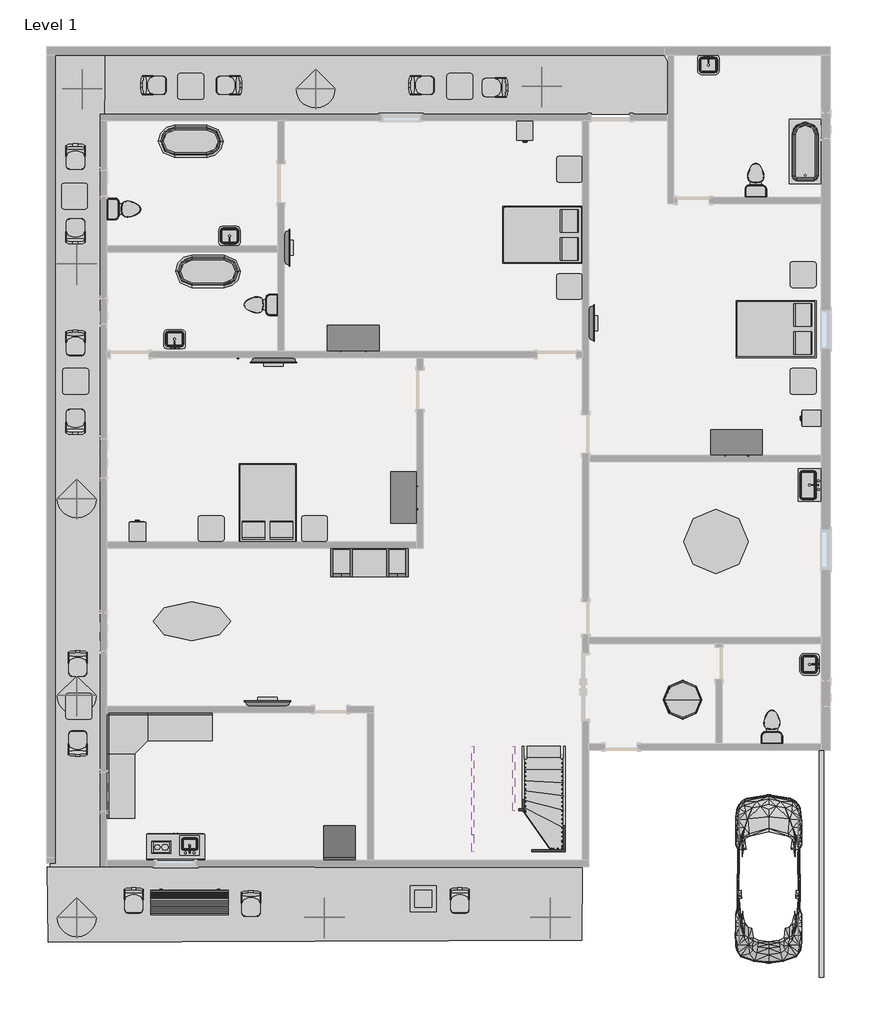
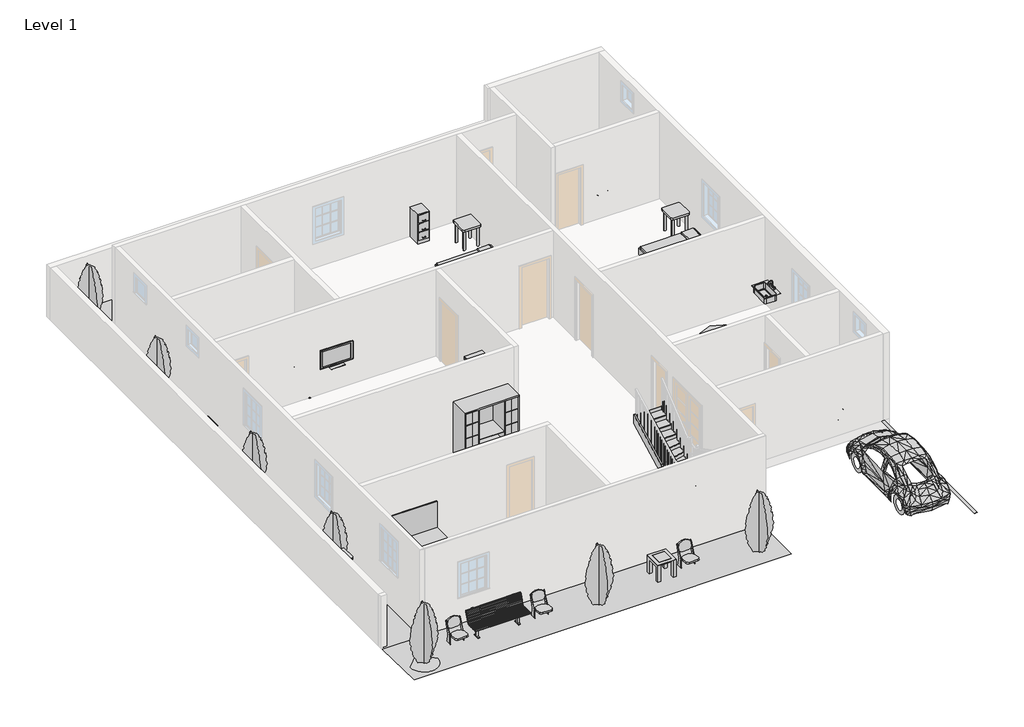
# One storey, part 3 of 3: 44 furniture elements, 18 flow terminals, 10 geographic elements, 8 members, 8 proxies, 1 stair flight.
"""IFC4 building model written with IfcOpenShell, lengths in millimetres."""

from ifc_helpers import new_model, si_unit, frame, origin, place, context, project, spatial, polyline, outline, extrude, triangles, transform, mapped, element, save
from components import proxy_fe84b772, proxy_844211aa, parking_space_9_x_18_90_deg_b8b21359, rpc_beetle_rpc_beetle_3ce7ba48, proxy_a13a33b2, flow_terminal_accce45a, flow_terminal_871c2e40, flow_terminal_38af2918, flow_terminal_62a433f7, toilet_domestic_3d_toilet_domestic_3d_f7549cf7, toilet_domestic_3d_toilet_domestic_3d_183bbd19, flow_terminal_b374fae2, tub_rectangular_3d_tub_rectangular_3d_ca47631e, furniture_c8abb964, furniture_552c1472, furniture_95afb093, furniture_9fa109b2, furniture_cf0b6580, furniture_3d1d9cbc, furniture_56245f3a, furniture_7a3aaa4f, furniture_b5c51a22, furniture_bbcc68ce, furniture_027a2ad9, furniture_bcf351fa, furniture_c80d6d9c, furniture_45e3acac, geographic_element_235d1464, rpc_tree_conifer_chinese_juniper_7_1b9786cd, stair_flight_703d0d0a

model = new_model("IFC4")

# Units and contexts
model_context = context("Model", 3, world=origin())
ifc_project = project(units=[si_unit("LENGTHUNIT", "METRE", prefix="MILLI")], contexts=[model_context])

# Site, building, storey
site = spatial("IfcSite", under=ifc_project)
building = spatial("IfcBuilding", under=site)
storey = spatial("IfcBuildingStorey", under=building, Name="Level 1", Elevation=0.0)

# Proxies
placement = place(None, origin())
element("IfcBuildingElementProxy", 1, Name="Building Element Proxy", at=placement, inside=storey, context=model_context, shape_type="Tessellation", body=[
    triangles([(-2806.8917519, -5680.9590546, 0.0), (-2820.1720459, -7388.5286636, 0.0), (-15417.9914612, -7439.908667, 0.0), (-15430.6918488, -5719.0590546, 0.0), (-15443.9724335, -5649.208667, 0.0)], [[5, 4, 1], [4, 5, 3], [2, 1, 4], [2, 4, 3]], closed=False),
])
element("IfcBuildingElementProxy", 2, Name="Building Element Proxy", at=placement, inside=storey, context=model_context, shape_type="Tessellation", body=[
    triangles([(-15354.4918488, -5446.0088608, 0.0), (-14186.0922363, -4794.6253647, 0.0), (-14084.355423, 13502.3909454, 0.0), (-15252.8922363, 13502.3909454, 0.0), (-14096.4674744, 13502.3909454, 0.0), (-14267.1105469, -5496.808667, 0.0), (-15252.8922363, -5496.808667, 0.0), (-14186.0922363, -5447.7901474, 0.0), (-14186.0922363, -5649.208667, 0.0), (-15366.6120392, -5649.208667, 0.0), (-15354.4918488, -5573.008667, 0.0)], [[10, 11, 1], [11, 10, 7], [4, 1, 2], [7, 1, 11], [2, 1, 7], [1, 4, 10], [10, 9, 7], [6, 9, 8], [9, 6, 7], [8, 9, 3], [6, 8, 2], [2, 3, 5], [3, 2, 8], [2, 7, 6], [5, 4, 2]], closed=False),
])
element("IfcBuildingElementProxy", 3, Name="Building Element Proxy", at=placement, inside=storey, context=model_context, shape_type="Tessellation", body=[
    triangles([(-14079.6975677, 13502.3909454, 0.0), (-876.4918488, 13502.3909454, 0.0), (-800.2918488, 12105.391333, 0.0), (-14186.0922363, 12105.391333, 0.0), (-800.2918488, 13334.3035309, 0.0)], [[1, 4, 3], [2, 3, 5], [3, 2, 1]], closed=False),
])
proxy_shape = proxy_fe84b772(model_context)
element("IfcBuildingElementProxy", 4, Name="Cook Top-2 Unit : 12\" x 18\"", ObjectType="Cook Top-2 Unit : 12\" x 18\"", at=placement, inside=storey, context=model_context, shape_type="MappedRepresentation", body=[
    mapped(proxy_shape, transform((-12781.2166579, -5115.8089531, 0.0), x_axis=(0.0, -1.0000000000000004, 0.0), y_axis=(1.0000000000000004, 0.0, 0.0), z_axis=(0.0, 0.0, 1.0))),
])
proxy_2_shape = proxy_844211aa(model_context)
element("IfcBuildingElementProxy", 5, Name="Kitchenette - Small : 54\"", ObjectType="Kitchenette - Small : 54\"", at=placement, inside=storey, context=model_context, shape_type="MappedRepresentation", body=[
    mapped(proxy_2_shape, transform((-12389.3541574, -5496.8089531, 0.0), x_axis=(-1.0000000000000004, 0.0, 0.0), y_axis=(0.0, -1.0000000000000004, 0.0), z_axis=(0.0, 0.0, 1.0))),
])
parking_space_9_x_18_90_deg_shape = parking_space_9_x_18_90_deg_b8b21359(model_context)
element("IfcBuildingElementProxy", 6, Name="Parking Space : 9' x 18' - 90 deg", ObjectType="Parking Space : 9' x 18' - 90 deg", at=placement, inside=storey, context=model_context, shape_type="MappedRepresentation", body=[
    mapped(parking_space_9_x_18_90_deg_shape, transform((2831.9081377, -8265.4089531, 0.0), x_axis=(-1.0000000000000004, 0.0, 0.0), y_axis=(0.0, -1.0000000000000004, 0.0), z_axis=(0.0, 0.0, 1.0))),
])
rpc_beetle_rpc_beetle_shape = rpc_beetle_rpc_beetle_3ce7ba48(model_context)
element("IfcBuildingElementProxy", 7, Name="RPC Beetle : RPC Beetle", ObjectType="RPC Beetle : RPC Beetle", at=placement, inside=storey, context=model_context, shape_type="MappedRepresentation", body=[
    mapped(rpc_beetle_rpc_beetle_shape, transform((1587.3081377, -7173.2089531, 0.0), x_axis=(1.0, 0.0, 0.0), y_axis=(0.0, 1.0, 0.0), z_axis=(0.0, 0.0, 1.0))),
])
proxy_3_shape = proxy_a13a33b2(model_context)
element("IfcBuildingElementProxy", 8, Name="Refrigerator : 30\" x 32\" RH", ObjectType="Refrigerator : 30\" x 32\" RH", at=placement, inside=storey, context=model_context, shape_type="MappedRepresentation", body=[
    mapped(proxy_3_shape, transform((-8539.3543623, -5078.9079246, 0.0), x_axis=(1.0, 0.0, 0.0), y_axis=(0.0, 1.0, 0.0), z_axis=(0.0, 0.0, 1.0))),
])

# Flow terminals
flow_terminal_shape = flow_terminal_accce45a(model_context)
element("IfcFlowTerminal", 9, ObjectType="Floor Drain - Round : 5\" Strainer - 2\" Drain", at=placement, inside=storey, context=model_context, shape_type="MappedRepresentation", body=[
    mapped(flow_terminal_shape, transform((-10934.8918623, 6517.3910469, 0.0), x_axis=(-1.0, 0.0, 0.0), y_axis=(0.0, 0.0, 1.0), z_axis=(0.0, 1.0, 0.0))),
])
element("IfcFlowTerminal", 10, ObjectType="Floor Drain - Round : 5\" Strainer - 2\" Drain", at=placement, inside=storey, context=model_context, shape_type="MappedRepresentation", body=[
    mapped(flow_terminal_shape, transform((-10528.4918623, 6695.1910469, 0.0), x_axis=(1.0, 0.0, 0.0), y_axis=(0.0, 1.0, 0.0), z_axis=(0.0, 0.0, 1.0))),
])
element("IfcFlowTerminal", 11, ObjectType="Floor Drain - Round : 5\" Strainer - 2\" Drain", at=placement, inside=storey, context=model_context, shape_type="MappedRepresentation", body=[
    mapped(flow_terminal_shape, transform((-13500.2918623, 11190.9910469, 0.0), x_axis=(1.0, 0.0, 0.0), y_axis=(0.0, 1.0, 0.0), z_axis=(0.0, 0.0, 1.0))),
])
element("IfcFlowTerminal", 12, ObjectType="Floor Drain - Round : 5\" Strainer - 2\" Drain", at=placement, inside=storey, context=model_context, shape_type="MappedRepresentation", body=[
    mapped(flow_terminal_shape, transform((1815.9081377, 10378.1910469, 0.0), x_axis=(1.0, 0.0, 0.0), y_axis=(0.0, 1.0, 0.0), z_axis=(0.0, 0.0, 1.0))),
])
element("IfcFlowTerminal", 13, ObjectType="Floor Drain - Round : 5\" Strainer - 2\" Drain", at=placement, inside=storey, context=model_context, shape_type="MappedRepresentation", body=[
    mapped(flow_terminal_shape, transform((2302.2903293, -2187.6431505, 0.0), x_axis=(1.0, 0.0, 0.0), y_axis=(0.0, 1.0, 0.0), z_axis=(0.0, 0.0, 1.0))),
])
flow_terminal_2_shape = flow_terminal_871c2e40(model_context)
element("IfcFlowTerminal", 14, ObjectType="Sink Kitchen-Island : 18\" x 18\"", at=placement, inside=storey, context=model_context, shape_type="MappedRepresentation", body=[
    mapped(flow_terminal_2_shape, transform((-12062.2026218, -5151.563552, 0.0), x_axis=(-1.0000000000000004, 0.0, 0.0), y_axis=(0.0, -1.0000000000000004, 0.0), z_axis=(0.0, 0.0, 1.0))),
])
flow_terminal_3_shape = flow_terminal_38af2918(model_context)
element("IfcFlowTerminal", 15, ObjectType="Sink Kitchen-Single : 30\" x 21\"", at=placement, inside=storey, context=model_context, shape_type="MappedRepresentation", body=[
    mapped(flow_terminal_3_shape, transform((2550.1627366, 3370.7802875, 0.0), x_axis=(0.0, -1.0000000000000004, 0.0), y_axis=(1.0000000000000004, 0.0, 0.0), z_axis=(0.0, 0.0, 1.0))),
])
flow_terminal_4_shape = flow_terminal_62a433f7(model_context)
element("IfcFlowTerminal", 16, ObjectType="Sink Vanity-Square : 20\" x 18\"", at=placement, inside=storey, context=model_context, shape_type="MappedRepresentation", body=[
    mapped(flow_terminal_4_shape, transform((-11122.4026218, 9186.736448, 0.0), x_axis=(-0.9999999999999998, 0.0, 0.0), y_axis=(0.0, -0.9999999999999998, 0.0), z_axis=(0.0, 0.0, 1.0))),
])
element("IfcFlowTerminal", 17, ObjectType="Sink Vanity-Square : 20\" x 18\"", at=placement, inside=storey, context=model_context, shape_type="MappedRepresentation", body=[
    mapped(flow_terminal_4_shape, transform((-12417.8026218, 6748.336448, 0.0), x_axis=(-1.0000000000000002, 0.0, 0.0), y_axis=(0.0, -1.0000000000000002, 0.0), z_axis=(0.0, 0.0, 1.0))),
])
element("IfcFlowTerminal", 18, ObjectType="Sink Vanity-Square : 20\" x 18\"", at=placement, inside=storey, context=model_context, shape_type="MappedRepresentation", body=[
    mapped(flow_terminal_4_shape, transform((149.2188971, 13322.2456458, 0.0), x_axis=(1.0, 0.0, 0.0), y_axis=(0.0, 1.0, 0.0), z_axis=(0.0, 0.0, 1.0))),
])
element("IfcFlowTerminal", 19, ObjectType="Sink Vanity-Square : 20\" x 18\"", at=placement, inside=storey, context=model_context, shape_type="MappedRepresentation", body=[
    mapped(flow_terminal_4_shape, transform((2600.9627366, -858.3197125, 0.0), x_axis=(0.0, -1.0000000000000004, 0.0), y_axis=(1.0000000000000004, 0.0, 0.0), z_axis=(0.0, 0.0, 1.0))),
])
toilet_domestic_3d_toilet_domestic_3d_shape = toilet_domestic_3d_toilet_domestic_3d_f7549cf7(model_context)
toilet_domestic_3d_toilet_domestic_3d_2_shape = toilet_domestic_3d_toilet_domestic_3d_183bbd19(model_context)
element("IfcFlowTerminal", 20, ObjectType="Toilet-Domestic-3D : Toilet-Domestic-3D", at=placement, inside=storey, context=model_context, shape_type="MappedRepresentation", body=[
    mapped(toilet_domestic_3d_toilet_domestic_3d_shape, transform((-10489.7878897, 7609.5910469, 0.0), x_axis=(0.0, -1.0, 0.0), y_axis=(1.0, 0.0, 0.0), z_axis=(0.0, 0.0, 1.0))),
    mapped(toilet_domestic_3d_toilet_domestic_3d_2_shape, transform((-10489.7878897, 7609.5910469, 0.0), x_axis=(0.0, -1.0, 0.0), y_axis=(1.0, 0.0, 0.0), z_axis=(0.0, 0.0, 1.0))),
])
element("IfcFlowTerminal", 21, ObjectType="Toilet-Domestic-3D : Toilet-Domestic-3D", at=placement, inside=storey, context=model_context, shape_type="MappedRepresentation", body=[
    mapped(toilet_domestic_3d_toilet_domestic_3d_shape, transform((-13538.995835, 9870.1910469, 0.0), x_axis=(0.0, 1.0000000000000002, 0.0), y_axis=(-1.0000000000000002, 0.0, 0.0), z_axis=(0.0, 0.0, 1.0))),
    mapped(toilet_domestic_3d_toilet_domestic_3d_2_shape, transform((-13538.995835, 9870.1910469, 0.0), x_axis=(0.0, 1.0000000000000002, 0.0), y_axis=(-1.0000000000000002, 0.0, 0.0), z_axis=(0.0, 0.0, 1.0))),
])
element("IfcFlowTerminal", 22, ObjectType="Toilet-Domestic-3D : Toilet-Domestic-3D", at=placement, inside=storey, context=model_context, shape_type="MappedRepresentation", body=[
    mapped(toilet_domestic_3d_toilet_domestic_3d_shape, transform((1283.1183774, 10644.2870743, 0.0), x_axis=(-1.0000000000000002, 0.0, 0.0), y_axis=(0.0, -1.0000000000000002, 0.0), z_axis=(0.0, 0.0, 1.0))),
    mapped(toilet_domestic_3d_toilet_domestic_3d_2_shape, transform((1283.1183774, 10644.2870743, 0.0), x_axis=(-1.0000000000000002, 0.0, 0.0), y_axis=(0.0, -1.0000000000000002, 0.0), z_axis=(0.0, 0.0, 1.0))),
])
element("IfcFlowTerminal", 23, ObjectType="Toilet-Domestic-3D : Toilet-Domestic-3D", at=placement, inside=storey, context=model_context, shape_type="MappedRepresentation", body=[
    mapped(toilet_domestic_3d_toilet_domestic_3d_shape, transform((1663.5081377, -2258.9129257, 0.0), x_axis=(-1.0000000000000004, 0.0, 0.0), y_axis=(0.0, -1.0000000000000004, 0.0), z_axis=(0.0, 0.0, 1.0))),
    mapped(toilet_domestic_3d_toilet_domestic_3d_2_shape, transform((1663.5081377, -2258.9129257, 0.0), x_axis=(-1.0000000000000004, 0.0, 0.0), y_axis=(0.0, -1.0000000000000004, 0.0), z_axis=(0.0, 0.0, 1.0))),
])
flow_terminal_5_shape = flow_terminal_b374fae2(model_context)
element("IfcFlowTerminal", 24, ObjectType="Tub-Free Standing-3D : 30\" x 60\"", at=placement, inside=storey, context=model_context, shape_type="MappedRepresentation", body=[
    mapped(flow_terminal_5_shape, transform((-11646.0918623, 8396.9910469, 0.0), x_axis=(0.0, -1.0000000000000004, 0.0), y_axis=(1.0000000000000004, 0.0, 0.0), z_axis=(0.0, 0.0, 1.0))),
])
element("IfcFlowTerminal", 25, ObjectType="Tub-Free Standing-3D : 30\" x 60\"", at=placement, inside=storey, context=model_context, shape_type="MappedRepresentation", body=[
    mapped(flow_terminal_5_shape, transform((-12052.4918623, 11470.3910469, 0.0), x_axis=(0.0, -1.0, 0.0), y_axis=(1.0, 0.0, 0.0), z_axis=(0.0, 0.0, 1.0))),
])
tub_rectangular_3d_tub_rectangular_3d_shape = tub_rectangular_3d_tub_rectangular_3d_ca47631e(model_context)
element("IfcFlowTerminal", 26, ObjectType="Tub-Rectangular-3D : Tub-Rectangular-3D", at=placement, inside=storey, context=model_context, shape_type="MappedRepresentation", body=[
    mapped(tub_rectangular_3d_tub_rectangular_3d_shape, transform((2933.5081377, 11577.6940156, 0.0), x_axis=(0.0, 1.0, 0.0), y_axis=(-1.0, 0.0, 0.0), z_axis=(0.0, 0.0, 1.0))),
])

# Furniture
furniture_shape = furniture_c8abb964(model_context)
element("IfcFurniture", 27, ObjectType="Bed-Box : Double 53\" x 74\"", at=placement, inside=storey, context=model_context, shape_type="MappedRepresentation", body=[
    mapped(furniture_shape, transform((-3512.2623541, 9599.7435059, 0.0), x_axis=(0.0, -1.0, 0.0), y_axis=(1.0, 0.0, 0.0), z_axis=(0.0, 0.0, 1.0))),
])
element("IfcFurniture", 28, ObjectType="Bed-Box : Double 53\" x 74\"", at=placement, inside=storey, context=model_context, shape_type="MappedRepresentation", body=[
    mapped(furniture_shape, transform((-9899.3213705, 2685.7385879, 0.0), x_axis=(-1.0000000000000002, 0.0, 0.0), y_axis=(0.0, -1.0000000000000002, 0.0), z_axis=(0.0, 0.0, 1.0))),
])
element("IfcFurniture", 29, ObjectType="Bed-Box : Double 53\" x 74\"", at=placement, inside=storey, context=model_context, shape_type="MappedRepresentation", body=[
    mapped(furniture_shape, transform((1999.5376459, 7377.2435059, 0.0), x_axis=(0.0, -0.9999999999999998, 0.0), y_axis=(0.9999999999999998, 0.0, 0.0), z_axis=(0.0, 0.0, 1.0))),
])
furniture_2_shape = furniture_552c1472(model_context)
element("IfcFurniture", 30, ObjectType="Cabinet-File 3 Drawer.0001 : 15\" x 18\"", at=placement, inside=storey, context=model_context, shape_type="MappedRepresentation", body=[
    mapped(furniture_2_shape, transform((-13437.6883094, 2108.0567468, 0.0), x_axis=(-1.0, 0.0, 0.0), y_axis=(0.0, -1.0, 0.0), z_axis=(0.0, 0.0, 1.0))),
])
element("IfcFurniture", 31, ObjectType="Cabinet-File 3 Drawer.0001 : 15\" x 18\"", at=placement, inside=storey, context=model_context, shape_type="MappedRepresentation", body=[
    mapped(furniture_2_shape, transform((-4037.8954153, 11866.525347, 0.0), x_axis=(1.0, 0.0, 0.0), y_axis=(0.0, 1.0, 0.0), z_axis=(0.0, 0.0, 1.0))),
])
element("IfcFurniture", 32, ObjectType="Cabinet-File 3 Drawer.0001 : 15\" x 18\"", at=placement, inside=storey, context=model_context, shape_type="MappedRepresentation", body=[
    mapped(furniture_2_shape, transform((2745.4424378, 4801.9945999, 0.0), x_axis=(0.0, -1.0, 0.0), y_axis=(1.0, 0.0, 0.0), z_axis=(0.0, 0.0, 1.0))),
])
furniture_3_shape = furniture_95afb093(model_context)
element("IfcFurniture", 33, ObjectType="Counter Top w Sink Hole : 24\" Depth", at=placement, inside=storey, context=model_context, shape_type="MappedRepresentation", body=[
    mapped(furniture_3_shape, transform((-12922.7541574, -5496.8089531, 0.0), x_axis=(-1.0000000000000004, 0.0, 0.0), y_axis=(0.0, -1.0000000000000004, 0.0), z_axis=(0.0, 0.0, 1.0))),
])
furniture_4_shape = furniture_9fa109b2(model_context)
element("IfcFurniture", 34, ObjectType="Dresser : 48\" x 72\" x 24\"", at=placement, inside=storey, context=model_context, shape_type="MappedRepresentation", body=[
    mapped(furniture_4_shape, transform((-7947.8986025, 7185.354001, 0.0), x_axis=(1.0, 0.0, 0.0), y_axis=(0.0, 1.0, 0.0), z_axis=(0.0, 0.0, 1.0))),
])
element("IfcFurniture", 35, ObjectType="Dresser : 48\" x 72\" x 24\"", at=placement, inside=storey, context=model_context, shape_type="MappedRepresentation", body=[
    mapped(furniture_4_shape, transform((-7386.4548164, 3332.1843067, 0.0), x_axis=(0.0, 1.0000000000000002, 0.0), y_axis=(-1.0000000000000002, 0.0, 0.0), z_axis=(0.0, 0.0, 1.0))),
])
element("IfcFurniture", 36, ObjectType="Dresser : 48\" x 72\" x 24\"", at=placement, inside=storey, context=model_context, shape_type="MappedRepresentation", body=[
    mapped(furniture_4_shape, transform((1094.5013975, 4721.554001, 0.0), x_axis=(1.0, 0.0, 0.0), y_axis=(0.0, 1.0, 0.0), z_axis=(0.0, 0.0, 1.0))),
])
furniture_5_shape = furniture_cf0b6580(model_context)
element("IfcFurniture", 37, ObjectType="Entertainment Center : 72\" x 72\" x 24\"", at=placement, inside=storey, context=model_context, shape_type="MappedRepresentation", body=[
    mapped(furniture_5_shape, transform((-7836.0918623, 1970.7910469, 0.0), x_axis=(1.0, 0.0, 0.0), y_axis=(0.0, 1.0, 0.0), z_axis=(0.0, 0.0, 1.0))),
])
furniture_6_shape = furniture_3d1d9cbc(model_context)
element("IfcFurniture", 38, ObjectType="Seating-Auditorium : 18\" x 24\" x 30\"", at=placement, inside=storey, context=model_context, shape_type="MappedRepresentation", body=[
    mapped(furniture_6_shape, transform((-4674.4164525, 12579.6631781, 0.0), x_axis=(0.0, 1.0000000000000009, 0.0), y_axis=(-1.0000000000000009, 0.0, 0.0), z_axis=(0.0, 0.0, 1.0))),
])
element("IfcFurniture", 39, ObjectType="Seating-Auditorium : 18\" x 24\" x 30\"", at=placement, inside=storey, context=model_context, shape_type="MappedRepresentation", body=[
    mapped(furniture_6_shape, transform((-6806.7672722, 12951.9189158, 0.0), x_axis=(0.0, -1.0000000000000004, 0.0), y_axis=(1.0000000000000004, 0.0, 0.0), z_axis=(0.0, 0.0, 1.0))),
])
element("IfcFurniture", 40, ObjectType="Seating-Auditorium : 18\" x 24\" x 30\"", at=placement, inside=storey, context=model_context, shape_type="MappedRepresentation", body=[
    mapped(furniture_6_shape, transform((-13131.3672722, 12951.9189158, 0.0), x_axis=(0.0, -1.0, 0.0), y_axis=(1.0, 0.0, 0.0), z_axis=(0.0, 0.0, 1.0))),
])
element("IfcFurniture", 41, ObjectType="Seating-Auditorium : 18\" x 24\" x 30\"", at=placement, inside=storey, context=model_context, shape_type="MappedRepresentation", body=[
    mapped(furniture_6_shape, transform((-10948.2164525, 12630.4631781, 0.0), x_axis=(0.0, 1.0, 0.0), y_axis=(-1.0, 0.0, 0.0), z_axis=(0.0, 0.0, 1.0))),
])
element("IfcFurniture", 42, ObjectType="Seating-Auditorium : 18\" x 24\" x 30\"", at=placement, inside=storey, context=model_context, shape_type="MappedRepresentation", body=[
    mapped(furniture_6_shape, transform((-14609.5639935, 11304.6664567, 0.0), x_axis=(-1.0000000000000004, 0.0, 0.0), y_axis=(0.0, -1.0000000000000004, 0.0), z_axis=(0.0, 0.0, 1.0))),
])
element("IfcFurniture", 43, ObjectType="Seating-Auditorium : 18\" x 24\" x 30\"", at=placement, inside=storey, context=model_context, shape_type="MappedRepresentation", body=[
    mapped(furniture_6_shape, transform((-14931.0197312, 9146.9156371, 0.0), x_axis=(1.0000000000000004, 0.0, 0.0), y_axis=(0.0, 1.0000000000000004, 0.0), z_axis=(0.0, 0.0, 1.0))),
])
element("IfcFurniture", 44, ObjectType="Seating-Auditorium : 18\" x 24\" x 30\"", at=placement, inside=storey, context=model_context, shape_type="MappedRepresentation", body=[
    mapped(furniture_6_shape, transform((-14609.5639935, 6910.4664567, 0.0), x_axis=(-1.0000000000000004, 0.0, 0.0), y_axis=(0.0, -1.0000000000000004, 0.0), z_axis=(0.0, 0.0, 1.0))),
])
element("IfcFurniture", 45, ObjectType="Seating-Auditorium : 18\" x 24\" x 30\"", at=placement, inside=storey, context=model_context, shape_type="MappedRepresentation", body=[
    mapped(furniture_6_shape, transform((-14931.0197312, 4651.1156371, 0.0), x_axis=(1.0, 0.0, 0.0), y_axis=(0.0, 1.0, 0.0), z_axis=(0.0, 0.0, 1.0))),
])
element("IfcFurniture", 46, ObjectType="Seating-Auditorium : 18\" x 24\" x 30\"", at=placement, inside=storey, context=model_context, shape_type="MappedRepresentation", body=[
    mapped(furniture_6_shape, transform((-14558.7639935, -658.7335433, 0.0), x_axis=(-1.0000000000000004, 0.0, 0.0), y_axis=(0.0, -1.0000000000000004, 0.0), z_axis=(0.0, 0.0, 1.0))),
])
element("IfcFurniture", 47, ObjectType="Seating-Auditorium : 18\" x 24\" x 30\"", at=placement, inside=storey, context=model_context, shape_type="MappedRepresentation", body=[
    mapped(furniture_6_shape, transform((-14880.2197312, -2943.4843629, 0.0), x_axis=(1.0, 0.0, 0.0), y_axis=(0.0, 1.0, 0.0), z_axis=(0.0, 0.0, 1.0))),
])
element("IfcFurniture", 48, ObjectType="Seating-Auditorium : 18\" x 24\" x 30\"", at=placement, inside=storey, context=model_context, shape_type="MappedRepresentation", body=[
    mapped(furniture_6_shape, transform((-13237.9639935, -6246.7335433, 0.0), x_axis=(-1.0000000000000004, 0.0, 0.0), y_axis=(0.0, -1.0000000000000004, 0.0), z_axis=(0.0, 0.0, 1.0))),
])
element("IfcFurniture", 49, ObjectType="Seating-Auditorium : 18\" x 24\" x 30\"", at=placement, inside=storey, context=model_context, shape_type="MappedRepresentation", body=[
    mapped(furniture_6_shape, transform((-10469.3639935, -6322.9335433, 0.0), x_axis=(-1.0000000000000004, 0.0, 0.0), y_axis=(0.0, -1.0000000000000004, 0.0), z_axis=(0.0, 0.0, 1.0))),
])
element("IfcFurniture", 50, ObjectType="Seating-Auditorium : 18\" x 24\" x 30\"", at=placement, inside=storey, context=model_context, shape_type="MappedRepresentation", body=[
    mapped(furniture_6_shape, transform((-5541.7639935, -6246.7335433, 0.0), x_axis=(-1.0000000000000004, 0.0, 0.0), y_axis=(0.0, -1.0000000000000004, 0.0), z_axis=(0.0, 0.0, 1.0))),
])
furniture_7_shape = furniture_56245f3a(model_context)
element("IfcFurniture", 51, ObjectType="TV - Flat Screen : 32\"", at=placement, inside=storey, context=model_context, shape_type="MappedRepresentation", body=[
    mapped(furniture_7_shape, transform((-9784.1532387, 8959.735561, 914.4), x_axis=(0.0, 1.0000000000000009, 0.0), y_axis=(-1.0000000000000009, 0.0, 0.0), z_axis=(0.0, 0.0, 1.0))),
])
element("IfcFurniture", 52, ObjectType="TV - Flat Screen : 32\"", at=placement, inside=storey, context=model_context, shape_type="MappedRepresentation", body=[
    mapped(furniture_7_shape, transform((-2595.9532387, 7181.735561, 914.4), x_axis=(0.0, 1.0000000000000002, 0.0), y_axis=(-1.0000000000000002, 0.0, 0.0), z_axis=(0.0, 0.0, 1.0))),
])
furniture_8_shape = furniture_7a3aaa4f(model_context)
element("IfcFurniture", 53, ObjectType="TV - Flat Screen : 42\"", at=placement, inside=storey, context=model_context, shape_type="MappedRepresentation", body=[
    mapped(furniture_8_shape, transform((-10092.7473482, 6306.4524233, 914.4), x_axis=(1.0, 0.0, 0.0), y_axis=(0.0, 1.0, 0.0), z_axis=(0.0, 0.0, 1.0))),
])
element("IfcFurniture", 54, ObjectType="TV - Flat Screen : 42\"", at=placement, inside=storey, context=model_context, shape_type="MappedRepresentation", body=[
    mapped(furniture_8_shape, transform((-10242.4183437, -1806.0703294, 914.4), x_axis=(-1.0000000000000002, 0.0, 0.0), y_axis=(0.0, -1.0000000000000002, 0.0), z_axis=(0.0, 0.0, 1.0))),
])
furniture_9_shape = furniture_b5c51a22(model_context)
element("IfcFurniture", 55, ObjectType="Table-Coffee : 24\" x 24\" x 24\"", at=placement, inside=storey, context=model_context, shape_type="MappedRepresentation", body=[
    mapped(furniture_9_shape, transform((-6584.357629, -6506.4200309, 0.0), x_axis=(1.0, 0.0, 0.0), y_axis=(0.0, 1.0, 0.0), z_axis=(0.0, 0.0, 1.0))),
])
furniture_10_shape = furniture_bbcc68ce(model_context)
element("IfcFurniture", 56, ObjectType="Table-Dining Round w Chairs : 60\" Diameter", at=placement, inside=storey, context=model_context, shape_type="MappedRepresentation", body=[
    mapped(furniture_10_shape, transform((239.0261705, 2206.4697354, 0.0), x_axis=(1.0, 0.0, 0.0), y_axis=(0.0, 1.0, 0.0), z_axis=(0.0, 0.0, 1.0))),
])
furniture_11_shape = furniture_027a2ad9(model_context)
element("IfcFurniture", 57, ObjectType="Table-Ellipse : 72\" x 36\"", at=placement, inside=storey, context=model_context, shape_type="MappedRepresentation", body=[
    mapped(furniture_11_shape, transform((-12027.0918623, 141.9910469, 0.0), x_axis=(1.0, 0.0, 0.0), y_axis=(0.0, 1.0, 0.0), z_axis=(0.0, 0.0, 1.0))),
])
furniture_12_shape = furniture_bcf351fa(model_context)
element("IfcFurniture", 58, ObjectType="Table-End : 24\" x 24\"", at=placement, inside=storey, context=model_context, shape_type="MappedRepresentation", body=[
    mapped(furniture_12_shape, transform((-3420.2254926, 10657.5910469, 0.0), x_axis=(1.0, 0.0, 0.0), y_axis=(0.0, 1.0, 0.0), z_axis=(0.0, 0.0, 1.0))),
])
element("IfcFurniture", 59, ObjectType="Table-End : 24\" x 24\"", at=placement, inside=storey, context=model_context, shape_type="MappedRepresentation", body=[
    mapped(furniture_12_shape, transform((-3420.2254926, 7888.9910469, 0.0), x_axis=(1.0, 0.0, 0.0), y_axis=(0.0, 1.0, 0.0), z_axis=(0.0, 0.0, 1.0))),
])
element("IfcFurniture", 60, ObjectType="Table-End : 24\" x 24\"", at=placement, inside=storey, context=model_context, shape_type="MappedRepresentation", body=[
    mapped(furniture_12_shape, transform((-9440.0254926, 2173.9910469, 0.0), x_axis=(1.0, 0.0, 0.0), y_axis=(0.0, 1.0, 0.0), z_axis=(0.0, 0.0, 1.0))),
])
element("IfcFurniture", 61, ObjectType="Table-End : 24\" x 24\"", at=placement, inside=storey, context=model_context, shape_type="MappedRepresentation", body=[
    mapped(furniture_12_shape, transform((-11878.4254926, 2173.9910469, 0.0), x_axis=(1.0, 0.0, 0.0), y_axis=(0.0, 1.0, 0.0), z_axis=(0.0, 0.0, 1.0))),
])
element("IfcFurniture", 62, ObjectType="Table-End : 24\" x 24\"", at=placement, inside=storey, context=model_context, shape_type="MappedRepresentation", body=[
    mapped(furniture_12_shape, transform((2091.5745074, 8168.3910469, 0.0), x_axis=(1.0, 0.0, 0.0), y_axis=(0.0, 1.0, 0.0), z_axis=(0.0, 0.0, 1.0))),
])
element("IfcFurniture", 63, ObjectType="Table-End : 24\" x 24\"", at=placement, inside=storey, context=model_context, shape_type="MappedRepresentation", body=[
    mapped(furniture_12_shape, transform((2091.5745074, 5653.7910469, 0.0), x_axis=(1.0, 0.0, 0.0), y_axis=(0.0, 1.0, 0.0), z_axis=(0.0, 0.0, 1.0))),
])
element("IfcFurniture", 64, ObjectType="Table-End : 24\" x 24\"", at=placement, inside=storey, context=model_context, shape_type="MappedRepresentation", body=[
    mapped(furniture_12_shape, transform((-6011.0254926, 12613.3910469, 0.0), x_axis=(1.0, 0.0, 0.0), y_axis=(0.0, 1.0, 0.0), z_axis=(0.0, 0.0, 1.0))),
])
element("IfcFurniture", 65, ObjectType="Table-End : 24\" x 24\"", at=placement, inside=storey, context=model_context, shape_type="MappedRepresentation", body=[
    mapped(furniture_12_shape, transform((-12361.0254926, 12613.3910469, 0.0), x_axis=(1.0, 0.0, 0.0), y_axis=(0.0, 1.0, 0.0), z_axis=(0.0, 0.0, 1.0))),
])
element("IfcFurniture", 66, ObjectType="Table-End : 24\" x 24\"", at=placement, inside=storey, context=model_context, shape_type="MappedRepresentation", body=[
    mapped(furniture_12_shape, transform((-15104.2254926, 10022.5910469, 0.0), x_axis=(1.0, 0.0, 0.0), y_axis=(0.0, 1.0, 0.0), z_axis=(0.0, 0.0, 1.0))),
])
element("IfcFurniture", 67, ObjectType="Table-End : 24\" x 24\"", at=placement, inside=storey, context=model_context, shape_type="MappedRepresentation", body=[
    mapped(furniture_12_shape, transform((-15078.8254926, 5653.7910469, 0.0), x_axis=(1.0, 0.0, 0.0), y_axis=(0.0, 1.0, 0.0), z_axis=(0.0, 0.0, 1.0))),
])
element("IfcFurniture", 68, ObjectType="Table-End : 24\" x 24\"", at=placement, inside=storey, context=model_context, shape_type="MappedRepresentation", body=[
    mapped(furniture_12_shape, transform((-15002.6254926, -2017.0089531, 0.0), x_axis=(1.0, 0.0, 0.0), y_axis=(0.0, 1.0, 0.0), z_axis=(0.0, 0.0, 1.0))),
])
furniture_13_shape = furniture_c80d6d9c(model_context)
element("IfcFurniture", 69, ObjectType="Table-Round : 36\" Diameter", at=placement, inside=storey, context=model_context, shape_type="MappedRepresentation", body=[
    mapped(furniture_13_shape, transform((-444.6918623, -1712.2089531, 0.0), x_axis=(1.0, 0.0, 0.0), y_axis=(0.0, 1.0, 0.0), z_axis=(0.0, 0.0, 1.0))),
])
furniture_14_shape = furniture_45e3acac(model_context)
element("IfcFurniture", 70, ObjectType="Work Station Cubicle : 96\" x 96\"", at=placement, inside=storey, context=model_context, shape_type="MappedRepresentation", body=[
    mapped(furniture_14_shape, transform((-13901.9601101, -1521.9859455, 0.0), x_axis=(1.0, 0.0, 0.0), y_axis=(0.0, 1.0, 0.0), z_axis=(0.0, 0.0, 1.0))),
])

# Geographic elements
geographic_element_shape = geographic_element_235d1464(model_context)
element("IfcGeographicElement", 71, ObjectType="Park Bench : 72\"", at=placement, inside=storey, context=model_context, shape_type="MappedRepresentation", body=[
    mapped(geographic_element_shape, transform((-12077.8918623, -6462.0089531, 0.0), x_axis=(1.0, 0.0, 0.0), y_axis=(0.0, 1.0, 0.0), z_axis=(0.0, 0.0, 1.0))),
])
rpc_tree_conifer_chinese_juniper_7_shape = rpc_tree_conifer_chinese_juniper_7_1b9786cd(model_context)
element("IfcGeographicElement", 72, ObjectType="RPC Tree - Conifer : Chinese Juniper - 7'", at=placement, inside=storey, context=model_context, shape_type="MappedRepresentation", body=[
    mapped(rpc_tree_conifer_chinese_juniper_7_shape, transform((-3772.2885334, 12765.7910469, 0.0), x_axis=(1.0, 0.0, 0.0), y_axis=(0.0, 1.0, 0.0), z_axis=(0.0, 0.0, 1.0))),
])
element("IfcGeographicElement", 73, ObjectType="RPC Tree - Conifer : Chinese Juniper - 7'", at=placement, inside=storey, context=model_context, shape_type="MappedRepresentation", body=[
    mapped(rpc_tree_conifer_chinese_juniper_7_shape, transform((-9106.2885334, 12714.9910469, 0.0), x_axis=(1.0, 0.0, 0.0), y_axis=(0.0, 1.0, 0.0), z_axis=(0.0, 0.0, 1.0))),
])
element("IfcGeographicElement", 74, ObjectType="RPC Tree - Conifer : Chinese Juniper - 7'", at=placement, inside=storey, context=model_context, shape_type="MappedRepresentation", body=[
    mapped(rpc_tree_conifer_chinese_juniper_7_shape, transform((-14618.0885334, 12714.9910469, 0.0), x_axis=(1.0, 0.0, 0.0), y_axis=(0.0, 1.0, 0.0), z_axis=(0.0, 0.0, 1.0))),
])
element("IfcGeographicElement", 75, ObjectType="RPC Tree - Conifer : Chinese Juniper - 7'", at=placement, inside=storey, context=model_context, shape_type="MappedRepresentation", body=[
    mapped(rpc_tree_conifer_chinese_juniper_7_shape, transform((-14745.0885334, 8574.7910469, 0.0), x_axis=(1.0, 0.0, 0.0), y_axis=(0.0, 1.0, 0.0), z_axis=(0.0, 0.0, 1.0))),
])
element("IfcGeographicElement", 76, ObjectType="RPC Tree - Conifer : Chinese Juniper - 7'", at=placement, inside=storey, context=model_context, shape_type="MappedRepresentation", body=[
    mapped(rpc_tree_conifer_chinese_juniper_7_shape, transform((-14745.0885334, 3037.5910469, 0.0), x_axis=(1.0, 0.0, 0.0), y_axis=(0.0, 1.0, 0.0), z_axis=(0.0, 0.0, 1.0))),
])
element("IfcGeographicElement", 77, ObjectType="RPC Tree - Conifer : Chinese Juniper - 7'", at=placement, inside=storey, context=model_context, shape_type="MappedRepresentation", body=[
    mapped(rpc_tree_conifer_chinese_juniper_7_shape, transform((-14745.0885334, -1610.6089531, 0.0), x_axis=(1.0, 0.0, 0.0), y_axis=(0.0, 1.0, 0.0), z_axis=(0.0, 0.0, 1.0))),
])
element("IfcGeographicElement", 78, ObjectType="RPC Tree - Conifer : Chinese Juniper - 7'", at=placement, inside=storey, context=model_context, shape_type="MappedRepresentation", body=[
    mapped(rpc_tree_conifer_chinese_juniper_7_shape, transform((-14745.0885334, -6843.0089531, 0.0), x_axis=(1.0, 0.0, 0.0), y_axis=(0.0, 1.0, 0.0), z_axis=(0.0, 0.0, 1.0))),
])
element("IfcGeographicElement", 79, ObjectType="RPC Tree - Conifer : Chinese Juniper - 7'", at=placement, inside=storey, context=model_context, shape_type="MappedRepresentation", body=[
    mapped(rpc_tree_conifer_chinese_juniper_7_shape, transform((-8903.0885334, -6843.0089531, 0.0), x_axis=(1.0, 0.0, 0.0), y_axis=(0.0, 1.0, 0.0), z_axis=(0.0, 0.0, 1.0))),
])
element("IfcGeographicElement", 80, ObjectType="RPC Tree - Conifer : Chinese Juniper - 7'", at=placement, inside=storey, context=model_context, shape_type="MappedRepresentation", body=[
    mapped(rpc_tree_conifer_chinese_juniper_7_shape, transform((-3569.0885334, -6843.0089531, 0.0), x_axis=(1.0, 0.0, 0.0), y_axis=(0.0, 1.0, 0.0), z_axis=(0.0, 0.0, 1.0))),
])

# Members
element("IfcMember", 81, ObjectType="Stringer - 2\" Width", at=placement, inside=storey, context=model_context, shape_type="SweptSolid", body=[
    extrude(outline(polyline([(-2804.4089531, 229.639954), (-2804.4089531, 0.0), (-3024.1712707, 0.0), (-4891.8261448, 962.500629), (-4891.8261448, 1305.3956453), (-2804.4089531, 229.639954)])), frame((-3264.0918623, 0.0, 0.0), z_axis=(1.0, 0.0, 0.0), x_axis=(0.0, 1.0, 0.0)), (0.0, 0.0, 1.0), 50.8),
])
element("IfcMember", 82, ObjectType="Stringer - 2\" Width", at=placement, inside=storey, context=model_context, shape_type="SweptSolid", body=[
    extrude(outline(polyline([(-3264.0918623, -4891.8261448), (-3213.2918623, -4891.8261448), (-3213.2918623, -5246.540645), (-3264.0918623, -5246.540645), (-3264.0918623, -4891.8261448)])), frame((0.0, 0.0, 962.500629), z_axis=(0.0, 0.0, 1.0), x_axis=(1.0, 0.0, 0.0)), (0.0, 0.0, 1.0), 342.8950162),
])
element("IfcMember", 83, ObjectType="Stringer - 2\" Width", at=placement, inside=storey, context=model_context, shape_type="SweptSolid", body=[
    extrude(outline(polyline([(1000.5956453, -3213.2918623), (1289.0952212, -3213.2918623), (1969.9972697, -5335.311745), (1969.9972697, -5372.2918623), (1638.9682298, -5372.2918623), (1000.5956453, -3382.8143453), (1000.5956453, -3213.2918623)])), frame((0.0, -5297.340645, 0.0), z_axis=(0.0, 1.0, 0.0), x_axis=(0.0, 0.0, 1.0)), (0.0, 0.0, 1.0), 50.8),
])
element("IfcMember", 84, ObjectType="Stringer - 2\" Width", at=placement, inside=storey, context=model_context, shape_type="SweptSolid", body=[
    extrude(outline(polyline([(-5372.2918623, -5297.340645), (-5423.0918623, -5297.340645), (-5423.0918623, -4891.8261448), (-5372.2918623, -4891.8261448), (-5372.2918623, -5297.340645)])), frame((0.0, 0.0, 1649.8904473), z_axis=(0.0, 0.0, 1.0), x_axis=(1.0, 0.0, 0.0)), (0.0, 0.0, 1.0), 320.1068224),
])
element("IfcMember", 85, ObjectType="Stringer - 2\" Width", at=placement, inside=storey, context=model_context, shape_type="SweptSolid", body=[
    extrude(outline(polyline([(-4891.8261448, 1649.8904473), (-4891.8261448, 1969.9972697), (-2804.4089531, 3045.7529609), (-2804.4089531, 2725.6461385), (-4891.8261448, 1649.8904473)])), frame((-5423.0918623, 0.0, 0.0), z_axis=(1.0, 0.0, 0.0), x_axis=(0.0, 1.0, 0.0)), (0.0, 0.0, 1.0), 50.8),
])
element("IfcMember", 86, ObjectType="Stringer - 2\" Width", at=placement, inside=storey, context=model_context, shape_type="SweptSolid", body=[
    extrude(outline(polyline([(-2804.4089531, 176.1764461), (-2804.4089531, 0.0), (-3070.6705976, 0.0), (-4281.340645, 987.1410923), (-4281.340645, 1380.418648), (-2804.4089531, 176.1764461)])), frame((-4229.2918623, 0.0, 0.0), z_axis=(1.0, 0.0, 0.0), x_axis=(0.0, 1.0, 0.0)), (0.0, 0.0, 1.0), 50.8),
])
element("IfcMember", 87, ObjectType="Stringer - 2\" Width", at=placement, inside=storey, context=model_context, shape_type="SweptSolid", body=[
    extrude(outline(polyline([(1028.5617647, -4178.4918623), (1573.2682978, -4178.4918623), (1926.1409689, -4385.1289798), (1926.1409689, -4407.0918623), (1360.465107, -4407.0918623), (1028.5617647, -4212.7340796), (1028.5617647, -4178.4918623)])), frame((0.0, -4332.140645, 0.0), z_axis=(0.0, 1.0, 0.0), x_axis=(0.0, 0.0, 1.0)), (0.0, 0.0, 1.0), 50.8),
])
element("IfcMember", 88, ObjectType="Stringer - 2\" Width", at=placement, inside=storey, context=model_context, shape_type="SweptSolid", body=[
    extrude(outline(polyline([(-4332.140645, 1532.8634131), (-4332.140645, 1926.1409689), (-2804.4089531, 3171.8038432), (-2804.4089531, 2778.5262875), (-4332.140645, 1532.8634131)])), frame((-4457.8918623, 0.0, 0.0), z_axis=(1.0, 0.0, 0.0), x_axis=(0.0, 1.0, 0.0)), (0.0, 0.0, 1.0), 50.8),
])

# Stair flight
stair_flight_shape = stair_flight_703d0d0a(model_context)
element("IfcStairFlight", 89, ObjectType="2\" Tread 1\" Nosing 1/4\" Riser", at=placement, inside=storey, context=model_context, shape_type="MappedRepresentation", body=[
    mapped(stair_flight_shape, transform((0.0, 0.0, 0.0), x_axis=(1.0, 0.0, 0.0), y_axis=(0.0, 1.0, 0.0), z_axis=(0.0, 0.0, 1.0))),
])

save(model, "model.ifc")

# Revit data of these elements
# Type "Cook Top-2 Unit : 12\" x 18\""
#   Assembly Code = "E1090400"
#   Counter Height = 3' - 0"
#   Depth = 1' - 6"
#   Width = 1' - 0"
#   Burner Material = Steel, Chrome Plated
#   Cooktop Material = Steel, Polished
#   Default Elevation = 0
# Type "Kitchenette - Small : 54\""
#   Assembly Code = "E1090400"
#   Width = 4' - 6"
#   Height = 2' - 10 1/2"
#   Depth = 2' - 0"
#   Toe Depth = 0' - 3"
#   Toe Height = 0' - 3 1/2"
#   Cabinet Material = Cabinets
#   Door/Drawer Material = Cabinets
#   Handle Material = Cabinets - Handles
#   Default Elevation = 0
# Type "Parking Space : 9' x 18' - 90 deg"
#   Angle = 90.00°
#   Parking Length = 18' - 0"
#   Parking Width = 9' - 0"
#   pl = 18' - 0"
#   pw = 9' - 0"
# Type "RPC Beetle : RPC Beetle"
#   built-in parameter 1005195 = "RPC-16-0U6E-L4EG-ENH1-J3KF-SVEL-0TX4-C0"
#   Height = 0
# Type "Refrigerator : 30\" x 32\" RH"
#   Label = "REF."
#   Assembly Code = "E1090400"
#   Depth = 2' - 7 3/4"
#   Handle = 2' - 3"
#   Height = 5' - 10"
#   Rear Clearance = 0' - 2"
#   Top Door Height = 1' - 8"
#   Width = 2' - 5 3/8"
#   Material = Steel, Paint Finish, Ivory, Glossy
#   Default Elevation = 0
# Type "Floor Drain - Round : 5\" Strainer - 2\" Drain"
#   WFU = 2
#   Strainer Height = 0' - 3 1/4"
#   Strainer Radius = 0' - 2 1/2"
#   Strainer Diameter = 0' - 5"
#   Radius 6 = 0' - 0 5/8"
#   Radius 5 = 0' - 1 1/4"
#   Radius 4 = 0' - 1 7/8"
#   Radius 2 = 0' - 3.04167"
#   Radius 1 = 0' - 2.02083"
#   Radius 3 = 0' - 2 1/32"
#   Pipe Radius = 1"
#   Pipe Diameter = 2"
#   Height 2 = 0' - 0.725"
#   Height 1 = 0' - 1 13/16"
#   Body Radius = 0' - 4 1/16"
#   Body Height = 0' - 3 5/8"
#   Body Diameter = 0' - 8 1/8"
#   Drain Material = none
#   HWFU = 0
#   Default Elevation = 0
#   CWFU = 0
# Type "Sink Kitchen-Island : 18\" x 18\""
#   Assembly Code = "D2010410"
#   Counter Height = 3' - 0"
#   Depth = 1' - 6"
#   Width = 1' - 6"
#   Faucet Material = Steel, Polished
#   Sink Material = Steel, Polished
#   Default Elevation = 0
# Type "Sink Kitchen-Single : 30\" x 21\""
#   Assembly Code = "D2010410"
#   Counter Height = 3' - 0"
#   Depth = 1' - 9"
#   Width = 2' - 6"
#   Faucet Material = Steel, Polished
#   Sink Material = Steel, Polished
#   Default Elevation = 0
# Type "Sink Vanity-Square : 20\" x 18\""
#   Assembly Code = "D2010400"
#   Counter Height = 2' - 7"
#   Depth = 1' - 6"
#   Width = 1' - 8"
#   Basin Material = Porcelain, Linen
#   Faucet Material = Steel, Polished
#   Default Elevation = 0
# Type "Toilet-Domestic-3D : Toilet-Domestic-3D"
#   Assembly Code = "D2010110"
#   Toilet - Bowl/Basin Material = Porcelain, Linen
#   Toilet - Seat Material = Laminate, Linen, Matte
#   Default Elevation = 0
# Type "Tub-Free Standing-3D : 30\" x 60\""
#   Assembly Code = "D2010110"
#   Height = 1' - 6"
#   Length = 5' - 0"
#   Width = 2' - 6"
#   Tub Material = Porcelain, Ivory
#   Default Elevation = 0
# Type "Tub-Rectangular-3D : Tub-Rectangular-3D"
#   Assembly Code = "D2010500"
#   Depth = 2' - 6"
#   Height = 1' - 3"
#   Width = 5' - 0"
#   Tub Material = Porcelain, Ivory
#   Default Elevation = 0
# Type "Bed-Box : Double 53\" x 74\""
#   Assembly Code = "E2020200"
#   Length = 6' - 2"
#   Width = 4' - 5"
#   Frame Material = Birch
#   Mattress Material = Linen, White
#   Default Elevation = 0
# Type "Cabinet-File 3 Drawer.0001 : 15\" x 18\""
#   Assembly Code = "E2020200"
#   Depth = 1' - 6"
#   Height = 3' - 5"
#   Width = 1' - 3"
#   Cabinet Material = Steel, Paint Finish, Ivory, Glossy
#   Handle Material = Steel, Chrome Plated
#   Default Elevation = 0
# Type "Counter Top w Sink Hole : 24\" Depth"
#   Assembly Code = "C1030400"
#   Counter Thickness = 0' - 1 1/2"
#   Depth [instance default] = 2' - 1"
#   Height = 3' - 0"
#   Length [instance default] = 8' - 0"
#   Sink Location [instance default] = 2' - 0"
#   Sink Location To Wall [instance default] = 0' - 6"
#   Sink Opening Depth [instance default] = 1' - 3"
#   Sink Opening Width [instance default] = 2' - 3"
#   Counter Top Material = none
#   Default Elevation = 0
# Type "Dresser : 48\" x 72\" x 24\""
#   Assembly Code = "E2020200"
#   Depth = 2' - 0"
#   Height = 6' - 0"
#   Width = 4' - 0"
#   Dresser Material = Laminate - Ivory, Glossy
#   Drawer Material = Laminate, Ivory, Matte
#   Knob Material = Cherry
#   Default Elevation = 0
# Type "Entertainment Center : 72\" x 72\" x 24\""
#   Assembly Code = "E2020200"
#   Center Width = 2' - 8"
#   Depth = 2' - 0"
#   Height = 6' - 0"
#   Width = 6' - 0"
#   Material = none
#   Default Elevation = 0
# Type "Seating-Auditorium : 18\" x 24\" x 30\""
#   Assembly Code = "E2020200"
#   Seat Material = Linen, Beige
#   Frame Material = Steel, Paint Finish, Dark Gray, Matte
#   Default Elevation = 0
# Type "TV - Flat Screen : 32\""
#   SinAng = 0' - 0.0193"
#   L = 2' - 3.79372"
#   H = 1' - 3.6354"
#   Thickness = 0' - 4.33071"
#   Diagonal = 2' - 7.88976"
#   CosAng = 0' - 0.03431"
#   Stand [instance default] = yes
#   Default Elevation = 0
# Type "TV - Flat Screen : 42\""
#   SinAng = 0' - 0.0193"
#   L = 3' - 0.71517"
#   H = 1' - 8.65418"
#   Thickness = 0' - 4.33071"
#   Diagonal = 3' - 6.12598"
#   CosAng = 0' - 0.03431"
#   Stand [instance default] = yes
#   Default Elevation = 0
# Type "Table-Coffee : 24\" x 24\" x 24\""
#   Assembly Code = "E2020200"
#   Height = 2' - 0"
#   Length = 2' - 0"
#   Width = 2' - 0"
#   Top Material = none
#   Frame Material = none
#   Default Elevation = 0
# Type "Table-Dining Round w Chairs : 60\" Diameter"
#   Assembly Code = "E2020200"
#   Radius = 2' - 6"
#   Diameter = 5' - 0"
#   Height = 2' - 6"
#   Chairs = 6
#   Base Material = Pine
#   Top Material = Laminate, Linen, Matte
#   Default Elevation = 0
# Type "Table-Ellipse : 72\" x 36\""
#   Assembly Code = "E2020200"
#   Half Width = 1' - 6"
#   Half Length = 3' - 0"
#   Height = 2' - 6"
#   Length = 6' - 0"
#   Width = 3' - 0"
#   Base Material = Birch
#   Top Material = Laminate - Black
#   Default Elevation = 0
# Type "Table-End : 24\" x 24\""
#   Assembly Code = "E2020200"
#   Height = 2' - 6"
#   Length = 2' - 0"
#   Width = 2' - 0"
#   Base Material = Birch
#   Top Material = Laminate, Ivory, Matte
#   Default Elevation = 0
# Type "Table-Round : 36\" Diameter"
#   Assembly Code = "E2020200"
#   Base Radius = 0' - 10"
#   Height = 2' - 6"
#   Radius = 1' - 6"
#   Base Material = Steel, Chrome Plated
#   Top Material = Birch
#   Default Elevation = 0
# Type "Work Station Cubicle : 96\" x 96\""
#   Assembly Code = "E2020"
#   Desktop Height = 2' - 6"
#   Desktop1 Width = 2' - 0"
#   Desktop2 Width = 2' - 0"
#   Panel Height = 5' - 6"
#   Panel1 Length = 5' - 0"
#   Panel2 Length = 5' - 0"
#   Cube Panel Material = Textile - Light Gray
#   Work Top Material = Laminate, Ivory, Matte
#   Default Elevation = 0
# Type "Park Bench : 72\""
#   Length = 6' - 0"
#   Seat Material = Wood - Teak
#   Frame Material = Steel, Paint Finish, Dark Gray, Matte
# Type "RPC Tree - Conifer : Chinese Juniper - 7'"
#   built-in parameter 1005198 = "{2, 15},{39, RPC-16-FUM3-UUQ0-UBF0-N000-ST1L-LVER-AU},{1, 0},{1, 0},{2, 13},{1, 8},{5, Color},{1, 0},{1, 0},{3, 0.8},{3, 0.8},{3, 0.8},{1, 8},{7, BBoxMin},{1, 0},{1, 0},{1, 0},{1, 0},{1, 0},{1, 8},{7, BBoxMax},{1, 0},{1, 0},{1, 0},{1, 0},{1, 0},{2, 11},{9, RPCTypeId},{1, 0},{1, 0},{39, RPC-16-FUM3-UUQ0-UBF0-N000-ST1L-LVER-AU},{1, 6},{14, RPCPlantHeight},{1, 0},{1, 0},{1, 7},{2, 11},{7, keyword},{1, 0},{1, 0},{34, :RPCs:Trees [General]:Geometry:RPC},{2, 11},{8, category},{1, 0},{1, 0},{15, Trees [General]},{2, 11},{12, LocalizedUID},{1, 0},{1, 0},{15, Chinese Juniper},{2, 14},{6, Height},{1, 0},{1, 0},{1, 7},{1, 2},{16, Cast Reflections},{1, 0},{1, 0},{1, 0},{1, 2},{12, Cast Shadows},{1, 0},{1, 0},{1, 1},{1, 2},{9, Lock View},{1, 0},{1, 0},{1, 0},{1, 4},{5, ViewC},{1, 0},{1, 0},{1, 0},{21, assetlibrary_base.fbx},{1, 5},"
#   built-in parameter 1005195 = "RPC-16-FUM3-UUQ0-UBF0-N000-ST1L-LVER-AU"
#   Type Comments = "Chinese Juniper"
#   Assembly Code = "G2050500"
#   Height = 7' - 0"
#   Description = (empty or 0)
#   Default Elevation = 0
# Elements 1, 2, 3 (IfcBuildingElementProxy)
#   Material = none
#   Phase Created = New Construction
# Element 4 (IfcBuildingElementProxy, "Cook Top-2 Unit : 12\" x 18\"")
#   Phase Created = New Construction
#   Materials on its faces: "Steel, Chrome Plated", "Steel, Polished"
# Element 5 (IfcBuildingElementProxy, "Kitchenette - Small : 54\"")
#   Phase Created = New Construction
#   Materials on its faces: "Cabinets", "Cabinets - Handles"
# Element 6 (IfcBuildingElementProxy, "Parking Space : 9' x 18' - 90 deg")
#   Phase Created = New Construction
#   Materials on its faces: "Parking Stripe"
# Element 7 (IfcBuildingElementProxy, "RPC Beetle : RPC Beetle")
#   Phase Created = New Construction
# Element 8 (IfcBuildingElementProxy, "Refrigerator : 30\" x 32\" RH")
#   Phase Created = New Construction
#   Materials on its faces: "Steel, Paint Finish, Ivory, Glossy", "Steel, Chrome Plated"
# Element 9 (IfcFlowTerminal, "Floor Drain - Round : 5\" Strainer - 2\" Drain")
#   Mark = "18"
#   Phase Created = New Construction
# Element 10 (IfcFlowTerminal, "Floor Drain - Round : 5\" Strainer - 2\" Drain")
#   Mark = "19"
#   Phase Created = New Construction
# Element 11 (IfcFlowTerminal, "Floor Drain - Round : 5\" Strainer - 2\" Drain")
#   Mark = "20"
#   Phase Created = New Construction
# Element 12 (IfcFlowTerminal, "Floor Drain - Round : 5\" Strainer - 2\" Drain")
#   Mark = "21"
#   Phase Created = New Construction
# Element 13 (IfcFlowTerminal, "Floor Drain - Round : 5\" Strainer - 2\" Drain")
#   Mark = "22"
#   Phase Created = New Construction
# Element 14 (IfcFlowTerminal, "Sink Kitchen-Island : 18\" x 18\"")
#   Mark = "11"
#   Phase Created = New Construction
#   Materials on its faces: "Steel, Polished"
# Element 15 (IfcFlowTerminal, "Sink Kitchen-Single : 30\" x 21\"")
#   Mark = "15"
#   Phase Created = New Construction
#   Materials on its faces: "Steel, Polished"
# Element 16 (IfcFlowTerminal, "Sink Vanity-Square : 20\" x 18\"")
#   Mark = "2"
#   Phase Created = New Construction
#   Materials on its faces: "Porcelain, Linen", "Steel, Polished"
# Element 17 (IfcFlowTerminal, "Sink Vanity-Square : 20\" x 18\"")
#   Mark = "5"
#   Phase Created = New Construction
#   Materials on its faces: "Porcelain, Linen", "Steel, Polished"
# Element 18 (IfcFlowTerminal, "Sink Vanity-Square : 20\" x 18\"")
#   Mark = "14"
#   Phase Created = New Construction
#   Materials on its faces: "Porcelain, Linen", "Steel, Polished"
# Element 19 (IfcFlowTerminal, "Sink Vanity-Square : 20\" x 18\"")
#   Mark = "16"
#   Phase Created = New Construction
#   Materials on its faces: "Porcelain, Linen", "Steel, Polished"
# Element 20 (IfcFlowTerminal, "Toilet-Domestic-3D : Toilet-Domestic-3D")
#   Mark = "7"
#   Phase Created = New Construction
#   Materials on its faces: "Porcelain, Linen", "Laminate, Linen, Matte"
# Element 21 (IfcFlowTerminal, "Toilet-Domestic-3D : Toilet-Domestic-3D")
#   Mark = "9"
#   Phase Created = New Construction
#   Materials on its faces: "Porcelain, Linen", "Laminate, Linen, Matte"
# Element 22 (IfcFlowTerminal, "Toilet-Domestic-3D : Toilet-Domestic-3D")
#   Mark = "13"
#   Phase Created = New Construction
#   Materials on its faces: "Porcelain, Linen", "Laminate, Linen, Matte"
# Element 23 (IfcFlowTerminal, "Toilet-Domestic-3D : Toilet-Domestic-3D")
#   Mark = "17"
#   Phase Created = New Construction
#   Materials on its faces: "Porcelain, Linen", "Laminate, Linen, Matte"
# Element 24 (IfcFlowTerminal, "Tub-Free Standing-3D : 30\" x 60\"")
#   Mark = "6"
#   Phase Created = New Construction
#   Materials on its faces: "Porcelain, Ivory"
# Element 25 (IfcFlowTerminal, "Tub-Free Standing-3D : 30\" x 60\"")
#   Mark = "8"
#   Phase Created = New Construction
#   Materials on its faces: "Porcelain, Ivory"
# Element 26 (IfcFlowTerminal, "Tub-Rectangular-3D : Tub-Rectangular-3D")
#   Mark = "12"
#   Phase Created = New Construction
#   Materials on its faces: "Porcelain, Ivory"
# Elements 27, 28, 29 (IfcFurniture, "Bed-Box : Double 53\" x 74\"")
#   Phase Created = New Construction
#   Materials on its faces: "Birch", "Linen, White"
# Elements 30, 31, 32 (IfcFurniture, "Cabinet-File 3 Drawer.0001 : 15\" x 18\"")
#   Phase Created = New Construction
#   Materials on its faces: "Steel, Chrome Plated", "Steel, Paint Finish, Ivory, Glossy"
# Element 33 (IfcFurniture, "Counter Top w Sink Hole : 24\" Depth")
#   Sink Opening Depth = 1' - 3"
#   Sink Location To Wall = 0' - 6"
#   Length = 4' - 6"
#   Sink Location = 1' - 2"
#   Sink Opening Width = 1' - 4"
#   Depth = 2' - 0"
#   Phase Created = New Construction
#   Materials on its faces: "Counter Top"
# Elements 34, 35, 36 (IfcFurniture, "Dresser : 48\" x 72\" x 24\"")
#   Phase Created = New Construction
#   Materials on its faces: "Laminate, Ivory, Matte", "Cherry", "Laminate - Ivory, Glossy"
# Element 37 (IfcFurniture, "Entertainment Center : 72\" x 72\" x 24\"")
#   Phase Created = New Construction
#   Materials on its faces: "Steel, Chrome Plated", "Glass - Clear, Grey"
# Elements 38, 39, 40, 41, 42, 43, 44, 45, 46, 47, 48, 49, 50 (IfcFurniture, "Seating-Auditorium : 18\" x 24\" x 30\"")
#   Phase Created = New Construction
#   Materials on its faces: "Steel, Paint Finish, Dark Gray, Matte", "Linen, Beige"
# Elements 51, 52 (IfcFurniture, "TV - Flat Screen : 32\"")
#   Stand = yes
#   Phase Created = New Construction
#   Materials on its faces: "TV - Black", "TV - Glass", "TV - Screen"
# Elements 53, 54 (IfcFurniture, "TV - Flat Screen : 42\"")
#   Stand = yes
#   Phase Created = New Construction
#   Materials on its faces: "TV - Black", "TV - Glass", "TV - Screen"
# Element 55 (IfcFurniture, "Table-Coffee : 24\" x 24\" x 24\"")
#   Phase Created = New Construction
#   Materials on its faces: "Glass - Clear, Grey"
# Element 56 (IfcFurniture, "Table-Dining Round w Chairs : 60\" Diameter")
#   Phase Created = New Construction
#   Materials on its faces: "Pine", "Laminate, Linen, Matte"
# Element 57 (IfcFurniture, "Table-Ellipse : 72\" x 36\"")
#   Phase Created = New Construction
#   Materials on its faces: "Birch", "Laminate - Black"
# Elements 58, 59, 60, 61, 62, 63, 64, 65, 66, 67, 68 (IfcFurniture, "Table-End : 24\" x 24\"")
#   Phase Created = New Construction
#   Materials on its faces: "Laminate, Ivory, Matte", "Birch"
# Element 69 (IfcFurniture, "Table-Round : 36\" Diameter")
#   Phase Created = New Construction
#   Materials on its faces: "Steel, Chrome Plated", "Birch"
# Element 70 (IfcFurniture, "Work Station Cubicle : 96\" x 96\"")
#   Phase Created = New Construction
#   Materials on its faces: "Textile - Light Gray", "Laminate, Ivory, Matte"
# Element 71 (IfcGeographicElement, "Park Bench : 72\"")
#   Phase Created = New Construction
#   Materials on its faces: "Wood - Teak", "Steel, Paint Finish, Dark Gray, Matte"
# Elements 72, 73, 74, 75, 76, 77, 78, 79, 80 (IfcGeographicElement, "RPC Tree - Conifer : Chinese Juniper - 7'")
#   Phase Created = New Construction
# Elements 81, 82, 83, 84, 85, 86, 87, 88 (IfcMember, "Stringer - 2\" Width")
#   Phase Created = New Construction
# Element 89 (IfcStairFlight, "2\" Tread 1\" Nosing 1/4\" Riser")
#   Phase Created = New Construction
# Materials
#   "Steel, Chrome Plated": class "Metal", colour RGB 17 17 17, transparency 0, Description = "Chromiuim plated steel", Cost = 0
#   "Steel, Polished": class "Metal", colour RGB 57 57 57, transparency 0, Description = "Polished steel", Cost = 0
#   "Cabinets": colour RGB 249 249 249, transparency 0
#   "Cabinets - Handles": class "Metal", colour RGB 57 57 57, transparency 0
#   "Steel, Paint Finish, Ivory, Glossy": class "Metal", colour RGB 247 247 239, transparency 0, Description = "Steel, paint finish, ivory, glossy", Cost = 0
#   "Porcelain, Linen": class "Ceramic", colour RGB 249 239 230, transparency 0, Description = "Porcelain, linen", Cost = 0
#   "Laminate, Linen, Matte": class "Plastic", colour RGB 249 239 230, transparency 0, Description = "Plastic Laminate - Linen, Matte", Cost = 0
#   "Porcelain, Ivory": class "Ceramic", colour RGB 247 247 239, transparency 0, Description = "Porcelain, ivory", Cost = 0
#   "Birch": class "Wood", colour RGB 224 178 126, transparency 0, Description = "Betula Alleghaniensis", Cost = 0
#   "Linen, White": class "Textile", colour RGB 247 247 239, transparency 0, Description = "Linen, white", Cost = 0
#   "Laminate - Ivory, Glossy": colour RGB 247 247 239, transparency 0
#   "Laminate, Ivory, Matte": class "Plastic", colour RGB 247 247 239, transparency 0, Description = "Plastic Laminate - Ivory, Matte", Cost = 0
#   "Cherry": class "Wood", colour RGB 226 177 128, transparency 0, Description = "Prunus Serotina", Cost = 0
#   "Linen, Beige": class "Textile", colour RGB 249 239 230, transparency 0, Description = "Linen, beige", Cost = 0
#   "Steel, Paint Finish, Dark Gray, Matte": class "Metal", colour RGB 0 0 0, transparency 0, Description = "Steel, paint finish, dark gray, matte", Cost = 0
#   "Pine": class "Wood", colour RGB 223 192 134, transparency 0, Description = "Pinus Echinata", Cost = 0
#   "Laminate - Black": colour RGB 0 0 0, transparency 0
#   "Textile - Light Gray": class "Fabric", colour RGB 204 204 204, transparency 0
#   "Wood - Teak": class "Wood", colour RGB 120 73 19, transparency 0
#   "Parking Stripe": class "Paint", colour RGB 250 250 91, transparency 0
#   "Counter Top": class "Wood", colour RGB 226 177 128, transparency 0
#   "Glass - Clear, Grey": class "Glass", colour RGB 252 255 255, transparency 0.64
#   "TV - Black": colour RGB 49 49 49, transparency 0
#   "TV - Glass": colour RGB 157 157 157, transparency 0.9
#   "TV - Screen": colour RGB 0 0 0, transparency 0
